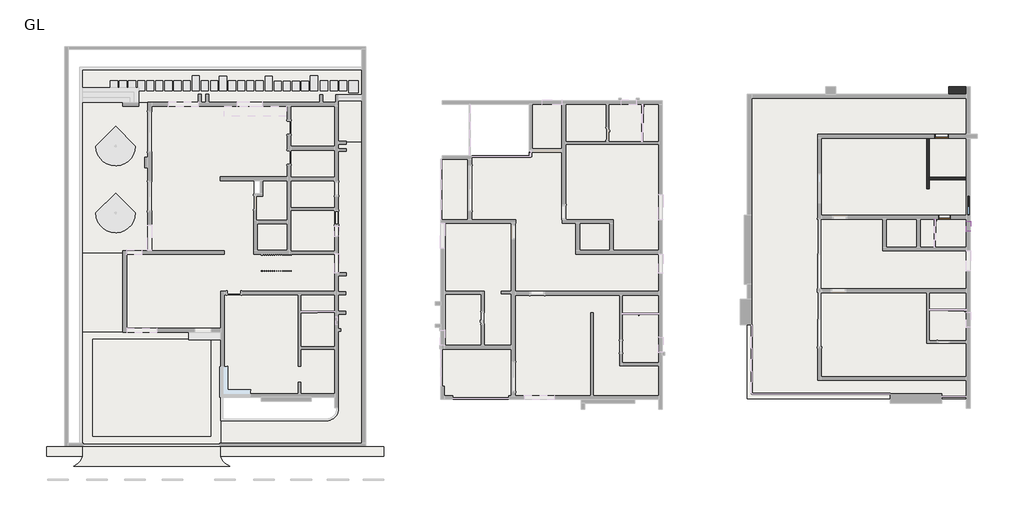
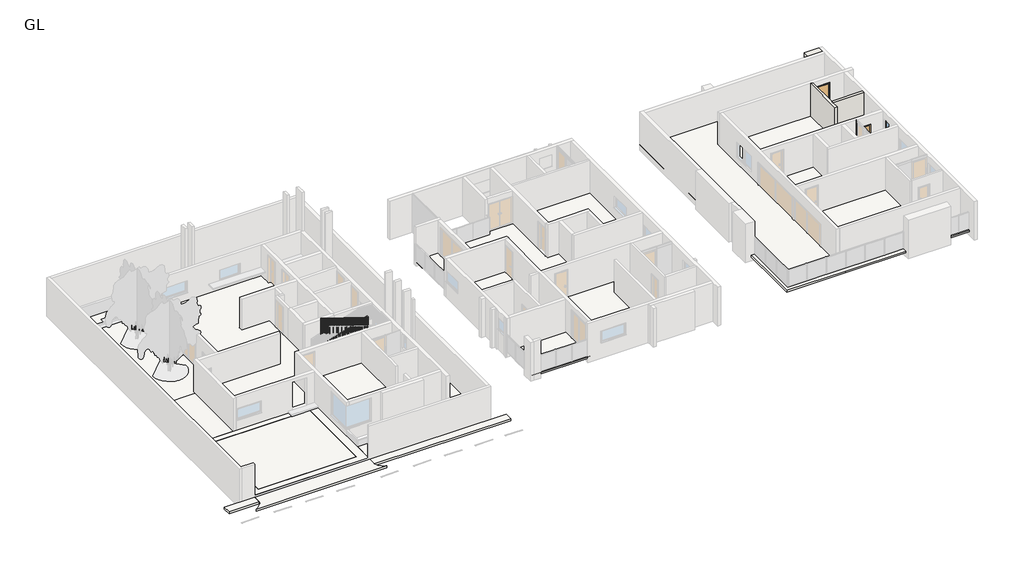
# One storey, part 5 of 6: 20 slabs, 3 walls, 2 doors, 2 members, 2 windows, 1 railing.
"""IFC4 building model written with IfcOpenShell, lengths in millimetres."""

from ifc_helpers import new_model, si_unit, point, frame, frame_2d, origin, origin_with_axes, place, context, project, spatial, polyline, circle_curve, trimmed, segment, composite_curve, outline, extrude, faceted_brep, transform, mapped, element, save
from components import door_b7cddb0a, doors_intsgl_2_5_5ac032e7, rectangular_mullion_30mm_square_28ebc8b3, rectangular_mullion_30mm_square_b4ecd99e, parametric_operable_sliding_window_6387_4_f716cbab, windows_sgl_plain_2_8d1346b0

model = new_model("IFC4")

# Units and contexts
model_context = context("Model", 3, world=origin())
ifc_project = project(units=[si_unit("LENGTHUNIT", "METRE", prefix="MILLI")], contexts=[model_context])

# Site, building, storey
site = spatial("IfcSite", under=ifc_project)
building = spatial("IfcBuilding", under=site)
storey = spatial("IfcBuildingStorey", under=building, Name="GL", Elevation=0.0)

# Doors
placement = place(None, origin())
door_shape = door_b7cddb0a(model_context)
element("IfcDoor", 1, ObjectType="Doors_IntSgl : 2'11\"", at=placement, inside=storey, context=model_context, shape_type="MappedRepresentation", body=[
    mapped(door_shape, transform((1570.3662427, 25098.2592769, 449.9570313), x_axis=(1.0, 0.0, 0.0), y_axis=(0.0, 1.0, 0.0), z_axis=(0.0, 0.0, 1.0))),
])
doors_intsgl_2_5_shape = doors_intsgl_2_5_5ac032e7(model_context)
element("IfcDoor", 2, ObjectType="Doors_IntSgl : 2.5'", at=placement, inside=storey, context=model_context, shape_type="MappedRepresentation", body=[
    mapped(doors_intsgl_2_5_shape, transform((1748.6476997, 20128.7664182, 449.9570313), x_axis=(1.0, 0.0, 0.0), y_axis=(0.0, 1.0, 0.0), z_axis=(0.0, 0.0, 1.0))),
])

# Members
rectangular_mullion_30mm_square_shape = rectangular_mullion_30mm_square_28ebc8b3(model_context)
element("IfcMember", 3, ObjectType="Rectangular Mullion : 30mm_Square", at=placement, inside=storey, context=model_context, shape_type="MappedRepresentation", body=[
    mapped(rectangular_mullion_30mm_square_shape, transform((1132.6976997, 20014.4664182, 3000.0), x_axis=(0.0, 1.0, 0.0), y_axis=(-1.0, 0.0, 0.0), z_axis=(0.0, 0.0, 1.0))),
])
rectangular_mullion_30mm_square_2_shape = rectangular_mullion_30mm_square_b4ecd99e(model_context)
element("IfcMember", 4, ObjectType="Rectangular Mullion : 30mm_Square", at=placement, inside=storey, context=model_context, shape_type="MappedRepresentation", body=[
    mapped(rectangular_mullion_30mm_square_2_shape, transform((1132.6976997, 20014.4664182, 2849.9570312), x_axis=(0.0, 1.0, 0.0), y_axis=(-1.0, 0.0, 0.0), z_axis=(0.0, 0.0, 1.0))),
])

# Railing
element("IfcRailing", 5, ObjectType="1100mm", at=placement, inside=storey, context=model_context, shape_type="SolidModel", body=[
    faceted_brep([(-40149.9681829, 16845.7531621, 1799.9767904), (-40149.9681829, 16845.7531621, 1747.4487757), (-40149.9681829, 16795.7531621, 1747.4487757), (-40149.9681829, 16795.7531621, 1799.9767904), (-36808.2681829, 16845.7531621, 2875.9675095), (-36758.2681829, 16845.7531621, 2839.538946), (-36758.2681829, 16795.7531621, 2839.538946), (-36808.2681829, 16795.7531621, 2875.9675095), (-36808.2681829, 16845.7531621, 2899.9878906), (-36758.2681829, 16845.7531621, 2849.9878906), (-36758.2681829, 16795.7531621, 2849.9878906), (-36808.2681829, 16795.7531621, 2899.9878906), (-36683.2681829, 16845.7531621, 2899.9878906), (-36683.2681829, 16845.7531621, 2849.9878906), (-36733.2681829, 16795.7531621, 2849.9878906), (-36733.2681829, 16795.7531621, 2899.9878906), (-36683.2681829, 16720.7531621, 2899.9878906), (-36683.2681829, 16720.7531621, 2849.9878906), (-36733.2681829, 16720.7531621, 2849.9878906), (-36733.2681829, 16720.7531621, 2899.9878906), (-36683.2681829, 16717.5531621, 2899.9878906), (-36683.2681829, 16667.5531621, 2849.9878906), (-36733.2681829, 16667.5531621, 2849.9878906), (-36733.2681829, 16717.5531621, 2899.9878906), (-36683.2681829, 16717.5531621, 3024.0092809), (-36683.2681829, 16667.5531621, 2974.0092809), (-36733.2681829, 16667.5531621, 2974.0092809), (-36733.2681829, 16717.5531621, 3024.0092809), (-36683.2681829, 16592.5531621, 3024.0092809), (-36683.2681829, 16592.5531621, 2974.0092809), (-36733.2681829, 16642.5531621, 2974.0092809), (-36733.2681829, 16642.5531621, 3024.0092809), (-36808.2681829, 16592.5531621, 3024.0092809), (-36816.1194278, 16592.5531621, 2974.0092809), (-36816.1194278, 16642.5531621, 2974.0092809), (-36808.2681829, 16642.5531621, 3024.0092809), (-40149.9681829, 16592.5531621, 4100.0), (-40149.9681829, 16642.5531621, 4100.0), (-40149.9681829, 16642.5531621, 4047.4719853), (-40149.9681829, 16592.5531621, 4047.4719853)], [[[0, 1, 2, 3]], [[1, 0, 4, 5]], [[2, 1, 5, 6]], [[3, 2, 6, 7]], [[0, 3, 7, 4]], [[5, 4, 8, 9]], [[6, 5, 9, 10]], [[7, 6, 10, 11]], [[4, 7, 11, 8]], [[9, 8, 12, 13]], [[10, 9, 13, 14]], [[11, 10, 14, 15]], [[8, 11, 15, 12]], [[13, 12, 16, 17]], [[14, 13, 17, 18]], [[15, 14, 18, 19]], [[12, 15, 19, 16]], [[17, 16, 20, 21]], [[18, 17, 21, 22]], [[19, 18, 22, 23]], [[16, 19, 23, 20]], [[21, 20, 24, 25]], [[22, 21, 25, 26]], [[23, 22, 26, 27]], [[20, 23, 27, 24]], [[25, 24, 28, 29]], [[26, 25, 29, 30]], [[27, 26, 30, 31]], [[24, 27, 31, 28]], [[29, 28, 32, 33]], [[30, 29, 33, 34]], [[31, 30, 34, 35]], [[28, 31, 35, 32]], [[36, 37, 38, 39]], [[33, 32, 36, 39]], [[34, 33, 39, 38]], [[35, 34, 38, 37]], [[32, 35, 37, 36]]]),
    extrude(outline(polyline([(2899.9989909, -40133.2681829), (4042.0947686, -40133.2681829), (4050.1444942, -40158.2681829), (2899.9989909, -40158.2681829), (2899.9989909, -40133.2681829)])), frame((0.0, 16605.0531621, 0.0), z_axis=(0.0, 1.0, 0.0), x_axis=(0.0, 0.0, 1.0)), (0.0, 0.0, 1.0), 25.0),
    extrude(outline(polyline([(2899.9989909, -40008.2681829), (4001.8461407, -40008.2681829), (4009.8958663, -40033.2681829), (2899.9989909, -40033.2681829), (2899.9989909, -40008.2681829)])), frame((0.0, 16605.0531621, 0.0), z_axis=(0.0, 1.0, 0.0), x_axis=(0.0, 0.0, 1.0)), (0.0, 0.0, 1.0), 25.0),
    extrude(outline(polyline([(2899.9989909, -39883.2681829), (3961.5975128, -39883.2681829), (3969.6472384, -39908.2681829), (2899.9989909, -39908.2681829), (2899.9989909, -39883.2681829)])), frame((0.0, 16605.0531621, 0.0), z_axis=(0.0, 1.0, 0.0), x_axis=(0.0, 0.0, 1.0)), (0.0, 0.0, 1.0), 25.0),
    extrude(outline(polyline([(2799.9979818, -39758.2681829), (3921.3488849, -39758.2681829), (3929.3986105, -39783.2681829), (2799.9979818, -39783.2681829), (2799.9979818, -39758.2681829)])), frame((0.0, 16605.0531621, 0.0), z_axis=(0.0, 1.0, 0.0), x_axis=(0.0, 0.0, 1.0)), (0.0, 0.0, 1.0), 25.0),
    extrude(outline(polyline([(2799.9979818, -39633.2681829), (3881.100257, -39633.2681829), (3889.1499826, -39658.2681829), (2799.9979818, -39658.2681829), (2799.9979818, -39633.2681829)])), frame((0.0, 16605.0531621, 0.0), z_axis=(0.0, 1.0, 0.0), x_axis=(0.0, 0.0, 1.0)), (0.0, 0.0, 1.0), 25.0),
    extrude(outline(polyline([(2699.9969727, -39508.2681829), (3840.8516291, -39508.2681829), (3848.9013546, -39533.2681829), (2699.9969727, -39533.2681829), (2699.9969727, -39508.2681829)])), frame((0.0, 16605.0531621, 0.0), z_axis=(0.0, 1.0, 0.0), x_axis=(0.0, 0.0, 1.0)), (0.0, 0.0, 1.0), 25.0),
    extrude(outline(polyline([(2699.9969727, -39383.2681829), (3800.6030011, -39383.2681829), (3808.6527267, -39408.2681829), (2699.9969727, -39408.2681829), (2699.9969727, -39383.2681829)])), frame((0.0, 16605.0531621, 0.0), z_axis=(0.0, 1.0, 0.0), x_axis=(0.0, 0.0, 1.0)), (0.0, 0.0, 1.0), 25.0),
    extrude(outline(polyline([(2699.9969727, -39258.2681829), (3760.3543732, -39258.2681829), (3768.4040988, -39283.2681829), (2699.9969727, -39283.2681829), (2699.9969727, -39258.2681829)])), frame((0.0, 16605.0531621, 0.0), z_axis=(0.0, 1.0, 0.0), x_axis=(0.0, 0.0, 1.0)), (0.0, 0.0, 1.0), 25.0),
    extrude(outline(polyline([(2599.9959635, -39133.2681829), (3720.1057453, -39133.2681829), (3728.1554709, -39158.2681829), (2599.9959635, -39158.2681829), (2599.9959635, -39133.2681829)])), frame((0.0, 16605.0531621, 0.0), z_axis=(0.0, 1.0, 0.0), x_axis=(0.0, 0.0, 1.0)), (0.0, 0.0, 1.0), 25.0),
    extrude(outline(polyline([(2599.9959635, -39008.2681829), (3679.8571174, -39008.2681829), (3687.906843, -39033.2681829), (2599.9959635, -39033.2681829), (2599.9959635, -39008.2681829)])), frame((0.0, 16605.0531621, 0.0), z_axis=(0.0, 1.0, 0.0), x_axis=(0.0, 0.0, 1.0)), (0.0, 0.0, 1.0), 25.0),
    extrude(outline(polyline([(2499.9949544, -38883.2681829), (3639.6084895, -38883.2681829), (3647.6582151, -38908.2681829), (2499.9949544, -38908.2681829), (2499.9949544, -38883.2681829)])), frame((0.0, 16605.0531621, 0.0), z_axis=(0.0, 1.0, 0.0), x_axis=(0.0, 0.0, 1.0)), (0.0, 0.0, 1.0), 25.0),
    extrude(outline(polyline([(2499.9949544, -38758.2681829), (3599.3598616, -38758.2681829), (3607.4095872, -38783.2681829), (2499.9949544, -38783.2681829), (2499.9949544, -38758.2681829)])), frame((0.0, 16605.0531621, 0.0), z_axis=(0.0, 1.0, 0.0), x_axis=(0.0, 0.0, 1.0)), (0.0, 0.0, 1.0), 25.0),
    extrude(outline(polyline([(2499.9949544, -38633.2681829), (3559.1112337, -38633.2681829), (3567.1609593, -38658.2681829), (2499.9949544, -38658.2681829), (2499.9949544, -38633.2681829)])), frame((0.0, 16605.0531621, 0.0), z_axis=(0.0, 1.0, 0.0), x_axis=(0.0, 0.0, 1.0)), (0.0, 0.0, 1.0), 25.0),
    extrude(outline(polyline([(2399.9939453, -38508.2681829), (3518.8626058, -38508.2681829), (3526.9123314, -38533.2681829), (2399.9939453, -38533.2681829), (2399.9939453, -38508.2681829)])), frame((0.0, 16605.0531621, 0.0), z_axis=(0.0, 1.0, 0.0), x_axis=(0.0, 0.0, 1.0)), (0.0, 0.0, 1.0), 25.0),
    extrude(outline(polyline([(2399.9939453, -38383.2681829), (3478.6139779, -38383.2681829), (3486.6637034, -38408.2681829), (2399.9939453, -38408.2681829), (2399.9939453, -38383.2681829)])), frame((0.0, 16605.0531621, 0.0), z_axis=(0.0, 1.0, 0.0), x_axis=(0.0, 0.0, 1.0)), (0.0, 0.0, 1.0), 25.0),
    extrude(outline(polyline([(2299.9929362, -38258.2681829), (3438.36535, -38258.2681829), (3446.4150755, -38283.2681829), (2299.9929362, -38283.2681829), (2299.9929362, -38258.2681829)])), frame((0.0, 16605.0531621, 0.0), z_axis=(0.0, 1.0, 0.0), x_axis=(0.0, 0.0, 1.0)), (0.0, 0.0, 1.0), 25.0),
    extrude(outline(polyline([(2299.9929362, -38133.2681829), (3398.116722, -38133.2681829), (3406.1664476, -38158.2681829), (2299.9929362, -38158.2681829), (2299.9929362, -38133.2681829)])), frame((0.0, 16605.0531621, 0.0), z_axis=(0.0, 1.0, 0.0), x_axis=(0.0, 0.0, 1.0)), (0.0, 0.0, 1.0), 25.0),
    extrude(outline(polyline([(2299.9929362, -38008.2681829), (3357.8680941, -38008.2681829), (3365.9178197, -38033.2681829), (2299.9929362, -38033.2681829), (2299.9929362, -38008.2681829)])), frame((0.0, 16605.0531621, 0.0), z_axis=(0.0, 1.0, 0.0), x_axis=(0.0, 0.0, 1.0)), (0.0, 0.0, 1.0), 25.0),
    extrude(outline(polyline([(2199.9919271, -37883.2681829), (3317.6194662, -37883.2681829), (3325.6691918, -37908.2681829), (2199.9919271, -37908.2681829), (2199.9919271, -37883.2681829)])), frame((0.0, 16605.0531621, 0.0), z_axis=(0.0, 1.0, 0.0), x_axis=(0.0, 0.0, 1.0)), (0.0, 0.0, 1.0), 25.0),
    extrude(outline(polyline([(2199.9919271, -37758.2681829), (3277.3708383, -37758.2681829), (3285.4205639, -37783.2681829), (2199.9919271, -37783.2681829), (2199.9919271, -37758.2681829)])), frame((0.0, 16605.0531621, 0.0), z_axis=(0.0, 1.0, 0.0), x_axis=(0.0, 0.0, 1.0)), (0.0, 0.0, 1.0), 25.0),
    extrude(outline(polyline([(2099.990918, -37633.2681829), (3237.1222104, -37633.2681829), (3245.171936, -37658.2681829), (2099.990918, -37658.2681829), (2099.990918, -37633.2681829)])), frame((0.0, 16605.0531621, 0.0), z_axis=(0.0, 1.0, 0.0), x_axis=(0.0, 0.0, 1.0)), (0.0, 0.0, 1.0), 25.0),
    extrude(outline(polyline([(2099.990918, -37508.2681829), (3196.8735825, -37508.2681829), (3204.9233081, -37533.2681829), (2099.990918, -37533.2681829), (2099.990918, -37508.2681829)])), frame((0.0, 16605.0531621, 0.0), z_axis=(0.0, 1.0, 0.0), x_axis=(0.0, 0.0, 1.0)), (0.0, 0.0, 1.0), 25.0),
    extrude(outline(polyline([(2099.990918, -37383.2681829), (3156.6249546, -37383.2681829), (3164.6746802, -37408.2681829), (2099.990918, -37408.2681829), (2099.990918, -37383.2681829)])), frame((0.0, 16605.0531621, 0.0), z_axis=(0.0, 1.0, 0.0), x_axis=(0.0, 0.0, 1.0)), (0.0, 0.0, 1.0), 25.0),
    extrude(outline(polyline([(1999.9899089, -37258.2681829), (3116.3763267, -37258.2681829), (3124.4260522, -37283.2681829), (1999.9899089, -37283.2681829), (1999.9899089, -37258.2681829)])), frame((0.0, 16605.0531621, 0.0), z_axis=(0.0, 1.0, 0.0), x_axis=(0.0, 0.0, 1.0)), (0.0, 0.0, 1.0), 25.0),
    extrude(outline(polyline([(1999.9899089, -37133.2681829), (3076.1276988, -37133.2681829), (3084.1774243, -37158.2681829), (1999.9899089, -37158.2681829), (1999.9899089, -37133.2681829)])), frame((0.0, 16605.0531621, 0.0), z_axis=(0.0, 1.0, 0.0), x_axis=(0.0, 0.0, 1.0)), (0.0, 0.0, 1.0), 25.0),
    extrude(outline(polyline([(1899.9888997, -37008.2681829), (3035.8790708, -37008.2681829), (3043.9287964, -37033.2681829), (1899.9888997, -37033.2681829), (1899.9888997, -37008.2681829)])), frame((0.0, 16605.0531621, 0.0), z_axis=(0.0, 1.0, 0.0), x_axis=(0.0, 0.0, 1.0)), (0.0, 0.0, 1.0), 25.0),
    extrude(outline(polyline([(1899.9888997, -36883.2681829), (2995.6304429, -36883.2681829), (3003.6801685, -36908.2681829), (1899.9888997, -36908.2681829), (1899.9888997, -36883.2681829)])), frame((0.0, 16605.0531621, 0.0), z_axis=(0.0, 1.0, 0.0), x_axis=(0.0, 0.0, 1.0)), (0.0, 0.0, 1.0), 25.0),
    extrude(outline(polyline([(-36758.2681829, 16630.0531621), (-36758.2681829, 16605.0531621), (-36783.2681829, 16605.0531621), (-36783.2681829, 16630.0531621), (-36758.2681829, 16630.0531621)])), frame((0.0, 0.0, 1899.9888997), z_axis=(0.0, 0.0, 1.0), x_axis=(1.0, 0.0, 0.0)), (0.0, 0.0, 1.0), 1074.0203811),
    extrude(outline(polyline([(-36720.7681829, 16645.7531621), (-36695.7681829, 16645.7531621), (-36695.7681829, 16620.7531621), (-36720.7681829, 16620.7531621), (-36720.7681829, 16645.7531621)])), frame((0.0, 0.0, 1799.9878906), z_axis=(0.0, 0.0, 1.0), x_axis=(1.0, 0.0, 0.0)), (0.0, 0.0, 1.0), 1174.0213903),
    extrude(outline(polyline([(-36720.7681829, 16770.7531621), (-36695.7681829, 16770.7531621), (-36695.7681829, 16745.7531621), (-36720.7681829, 16745.7531621), (-36720.7681829, 16770.7531621)])), frame((0.0, 0.0, 1799.9878906), z_axis=(0.0, 0.0, 1.0), x_axis=(1.0, 0.0, 0.0)), (0.0, 0.0, 1.0), 1050.0),
    extrude(outline(polyline([(-36724.9681829, 16808.2531621), (-36724.9681829, 16833.2531621), (-36699.9681829, 16833.2531621), (-36699.9681829, 16808.2531621), (-36724.9681829, 16808.2531621)])), frame((0.0, 0.0, 1799.9878906), z_axis=(0.0, 0.0, 1.0), x_axis=(1.0, 0.0, 0.0)), (0.0, 0.0, 1.0), 1050.0),
    extrude(outline(polyline([(2810.0125525, -36849.9681829), (1699.9868815, -36849.9681829), (1699.9868815, -36824.9681829), (2818.0622781, -36824.9681829), (2810.0125525, -36849.9681829)])), frame((0.0, 16808.2531621, 0.0), z_axis=(0.0, 1.0, 0.0), x_axis=(0.0, 0.0, 1.0)), (0.0, 0.0, 1.0), 25.0),
    extrude(outline(polyline([(2769.7639246, -36974.9681829), (1699.9868815, -36974.9681829), (1699.9868815, -36949.9681829), (2777.8136502, -36949.9681829), (2769.7639246, -36974.9681829)])), frame((0.0, 16808.2531621, 0.0), z_axis=(0.0, 1.0, 0.0), x_axis=(0.0, 0.0, 1.0)), (0.0, 0.0, 1.0), 25.0),
    extrude(outline(polyline([(2729.5152967, -37099.9681829), (1599.9858724, -37099.9681829), (1599.9858724, -37074.9681829), (2737.5650223, -37074.9681829), (2729.5152967, -37099.9681829)])), frame((0.0, 16808.2531621, 0.0), z_axis=(0.0, 1.0, 0.0), x_axis=(0.0, 0.0, 1.0)), (0.0, 0.0, 1.0), 25.0),
    extrude(outline(polyline([(2689.2666688, -37224.9681829), (1599.9858724, -37224.9681829), (1599.9858724, -37199.9681829), (2697.3163944, -37199.9681829), (2689.2666688, -37224.9681829)])), frame((0.0, 16808.2531621, 0.0), z_axis=(0.0, 1.0, 0.0), x_axis=(0.0, 0.0, 1.0)), (0.0, 0.0, 1.0), 25.0),
    extrude(outline(polyline([(2649.0180409, -37349.9681829), (1599.9858724, -37349.9681829), (1599.9858724, -37324.9681829), (2657.0677665, -37324.9681829), (2649.0180409, -37349.9681829)])), frame((0.0, 16808.2531621, 0.0), z_axis=(0.0, 1.0, 0.0), x_axis=(0.0, 0.0, 1.0)), (0.0, 0.0, 1.0), 25.0),
    extrude(outline(polyline([(2608.769413, -37474.9681829), (1499.9848633, -37474.9681829), (1499.9848633, -37449.9681829), (2616.8191385, -37449.9681829), (2608.769413, -37474.9681829)])), frame((0.0, 16808.2531621, 0.0), z_axis=(0.0, 1.0, 0.0), x_axis=(0.0, 0.0, 1.0)), (0.0, 0.0, 1.0), 25.0),
    extrude(outline(polyline([(2568.5207851, -37599.9681829), (1499.9848633, -37599.9681829), (1499.9848633, -37574.9681829), (2576.5705106, -37574.9681829), (2568.5207851, -37599.9681829)])), frame((0.0, 16808.2531621, 0.0), z_axis=(0.0, 1.0, 0.0), x_axis=(0.0, 0.0, 1.0)), (0.0, 0.0, 1.0), 25.0),
    extrude(outline(polyline([(2528.2721571, -37724.9681829), (1399.9838542, -37724.9681829), (1399.9838542, -37699.9681829), (2536.3218827, -37699.9681829), (2528.2721571, -37724.9681829)])), frame((0.0, 16808.2531621, 0.0), z_axis=(0.0, 1.0, 0.0), x_axis=(0.0, 0.0, 1.0)), (0.0, 0.0, 1.0), 25.0),
    extrude(outline(polyline([(2488.0235292, -37849.9681829), (1399.9838542, -37849.9681829), (1399.9838542, -37824.9681829), (2496.0732548, -37824.9681829), (2488.0235292, -37849.9681829)])), frame((0.0, 16808.2531621, 0.0), z_axis=(0.0, 1.0, 0.0), x_axis=(0.0, 0.0, 1.0)), (0.0, 0.0, 1.0), 25.0),
    extrude(outline(polyline([(2447.7749013, -37974.9681829), (1399.9838542, -37974.9681829), (1399.9838542, -37949.9681829), (2455.8246269, -37949.9681829), (2447.7749013, -37974.9681829)])), frame((0.0, 16808.2531621, 0.0), z_axis=(0.0, 1.0, 0.0), x_axis=(0.0, 0.0, 1.0)), (0.0, 0.0, 1.0), 25.0),
    extrude(outline(polyline([(2407.5262734, -38099.9681829), (1299.9828451, -38099.9681829), (1299.9828451, -38074.9681829), (2415.575999, -38074.9681829), (2407.5262734, -38099.9681829)])), frame((0.0, 16808.2531621, 0.0), z_axis=(0.0, 1.0, 0.0), x_axis=(0.0, 0.0, 1.0)), (0.0, 0.0, 1.0), 25.0),
    extrude(outline(polyline([(2367.2776455, -38224.9681829), (1299.9828451, -38224.9681829), (1299.9828451, -38199.9681829), (2375.3273711, -38199.9681829), (2367.2776455, -38224.9681829)])), frame((0.0, 16808.2531621, 0.0), z_axis=(0.0, 1.0, 0.0), x_axis=(0.0, 0.0, 1.0)), (0.0, 0.0, 1.0), 25.0),
    extrude(outline(polyline([(2327.0290176, -38349.9681829), (1199.9818359, -38349.9681829), (1199.9818359, -38324.9681829), (2335.0787432, -38324.9681829), (2327.0290176, -38349.9681829)])), frame((0.0, 16808.2531621, 0.0), z_axis=(0.0, 1.0, 0.0), x_axis=(0.0, 0.0, 1.0)), (0.0, 0.0, 1.0), 25.0),
    extrude(outline(polyline([(2286.7803897, -38474.9681829), (1199.9818359, -38474.9681829), (1199.9818359, -38449.9681829), (2294.8301153, -38449.9681829), (2286.7803897, -38474.9681829)])), frame((0.0, 16808.2531621, 0.0), z_axis=(0.0, 1.0, 0.0), x_axis=(0.0, 0.0, 1.0)), (0.0, 0.0, 1.0), 25.0),
    extrude(outline(polyline([(2246.5317618, -38599.9681829), (1199.9818359, -38599.9681829), (1199.9818359, -38574.9681829), (2254.5814873, -38574.9681829), (2246.5317618, -38599.9681829)])), frame((0.0, 16808.2531621, 0.0), z_axis=(0.0, 1.0, 0.0), x_axis=(0.0, 0.0, 1.0)), (0.0, 0.0, 1.0), 25.0),
    extrude(outline(polyline([(2206.2831339, -38724.9681829), (1099.9808268, -38724.9681829), (1099.9808268, -38699.9681829), (2214.3328594, -38699.9681829), (2206.2831339, -38724.9681829)])), frame((0.0, 16808.2531621, 0.0), z_axis=(0.0, 1.0, 0.0), x_axis=(0.0, 0.0, 1.0)), (0.0, 0.0, 1.0), 25.0),
    extrude(outline(polyline([(2166.0345059, -38849.9681829), (1099.9808268, -38849.9681829), (1099.9808268, -38824.9681829), (2174.0842315, -38824.9681829), (2166.0345059, -38849.9681829)])), frame((0.0, 16808.2531621, 0.0), z_axis=(0.0, 1.0, 0.0), x_axis=(0.0, 0.0, 1.0)), (0.0, 0.0, 1.0), 25.0),
    extrude(outline(polyline([(2125.785878, -38974.9681829), (999.9798177, -38974.9681829), (999.9798177, -38949.9681829), (2133.8356036, -38949.9681829), (2125.785878, -38974.9681829)])), frame((0.0, 16808.2531621, 0.0), z_axis=(0.0, 1.0, 0.0), x_axis=(0.0, 0.0, 1.0)), (0.0, 0.0, 1.0), 25.0),
    extrude(outline(polyline([(2085.5372501, -39099.9681829), (999.9798177, -39099.9681829), (999.9798177, -39074.9681829), (2093.5869757, -39074.9681829), (2085.5372501, -39099.9681829)])), frame((0.0, 16808.2531621, 0.0), z_axis=(0.0, 1.0, 0.0), x_axis=(0.0, 0.0, 1.0)), (0.0, 0.0, 1.0), 25.0),
    extrude(outline(polyline([(2045.2886222, -39224.9681829), (999.9798177, -39224.9681829), (999.9798177, -39199.9681829), (2053.3383478, -39199.9681829), (2045.2886222, -39224.9681829)])), frame((0.0, 16808.2531621, 0.0), z_axis=(0.0, 1.0, 0.0), x_axis=(0.0, 0.0, 1.0)), (0.0, 0.0, 1.0), 25.0),
    extrude(outline(polyline([(2005.0399943, -39349.9681829), (899.9788086, -39349.9681829), (899.9788086, -39324.9681829), (2013.0897199, -39324.9681829), (2005.0399943, -39349.9681829)])), frame((0.0, 16808.2531621, 0.0), z_axis=(0.0, 1.0, 0.0), x_axis=(0.0, 0.0, 1.0)), (0.0, 0.0, 1.0), 25.0),
    extrude(outline(polyline([(1964.7913664, -39474.9681829), (899.9788086, -39474.9681829), (899.9788086, -39449.9681829), (1972.841092, -39449.9681829), (1964.7913664, -39474.9681829)])), frame((0.0, 16808.2531621, 0.0), z_axis=(0.0, 1.0, 0.0), x_axis=(0.0, 0.0, 1.0)), (0.0, 0.0, 1.0), 25.0),
    extrude(outline(polyline([(1924.5427385, -39599.9681829), (799.9777995, -39599.9681829), (799.9777995, -39574.9681829), (1932.5924641, -39574.9681829), (1924.5427385, -39599.9681829)])), frame((0.0, 16808.2531621, 0.0), z_axis=(0.0, 1.0, 0.0), x_axis=(0.0, 0.0, 1.0)), (0.0, 0.0, 1.0), 25.0),
    extrude(outline(polyline([(1884.2941106, -39724.9681829), (799.9777995, -39724.9681829), (799.9777995, -39699.9681829), (1892.3438361, -39699.9681829), (1884.2941106, -39724.9681829)])), frame((0.0, 16808.2531621, 0.0), z_axis=(0.0, 1.0, 0.0), x_axis=(0.0, 0.0, 1.0)), (0.0, 0.0, 1.0), 25.0),
    extrude(outline(polyline([(1844.0454827, -39849.9681829), (799.9777995, -39849.9681829), (799.9777995, -39824.9681829), (1852.0952082, -39824.9681829), (1844.0454827, -39849.9681829)])), frame((0.0, 16808.2531621, 0.0), z_axis=(0.0, 1.0, 0.0), x_axis=(0.0, 0.0, 1.0)), (0.0, 0.0, 1.0), 25.0),
    extrude(outline(polyline([(1803.7968547, -39974.9681829), (699.9767904, -39974.9681829), (699.9767904, -39949.9681829), (1811.8465803, -39949.9681829), (1803.7968547, -39974.9681829)])), frame((0.0, 16808.2531621, 0.0), z_axis=(0.0, 1.0, 0.0), x_axis=(0.0, 0.0, 1.0)), (0.0, 0.0, 1.0), 25.0),
    extrude(outline(polyline([(1763.5482268, -40099.9681829), (699.9767904, -40099.9681829), (699.9767904, -40074.9681829), (1771.5979524, -40074.9681829), (1763.5482268, -40099.9681829)])), frame((0.0, 16808.2531621, 0.0), z_axis=(0.0, 1.0, 0.0), x_axis=(0.0, 0.0, 1.0)), (0.0, 0.0, 1.0), 25.0),
    extrude(outline(polyline([(-36720.7681829, 16630.0531621), (-36695.7681829, 16630.0531621), (-36695.7681829, 16605.0531621), (-36720.7681829, 16605.0531621), (-36720.7681829, 16630.0531621)])), frame((0.0, 0.0, 1799.9878906), z_axis=(0.0, 0.0, 1.0), x_axis=(1.0, 0.0, 0.0)), (0.0, 0.0, 1.0), 1174.0213903),
    extrude(outline(polyline([(-36720.7681829, 16808.2531621), (-36720.7681829, 16833.2531621), (-36695.7681829, 16833.2531621), (-36695.7681829, 16808.2531621), (-36720.7681829, 16808.2531621)])), frame((0.0, 0.0, 1799.9878906), z_axis=(0.0, 0.0, 1.0), x_axis=(1.0, 0.0, 0.0)), (0.0, 0.0, 1.0), 1050.0),
    extrude(outline(polyline([(2899.9989909, -40124.9681829), (4039.4222597, -40124.9681829), (4047.4719853, -40149.9681829), (2899.9989909, -40149.9681829), (2899.9989909, -40124.9681829)])), frame((0.0, 16605.0531621, 0.0), z_axis=(0.0, 1.0, 0.0), x_axis=(0.0, 0.0, 1.0)), (0.0, 0.0, 1.0), 25.0),
    extrude(outline(polyline([(1747.4487757, -40149.9681829), (699.9767904, -40149.9681829), (699.9767904, -40124.9681829), (1755.4985013, -40124.9681829), (1747.4487757, -40149.9681829)])), frame((0.0, 16808.2531621, 0.0), z_axis=(0.0, 1.0, 0.0), x_axis=(0.0, 0.0, 1.0)), (0.0, 0.0, 1.0), 25.0),
])

# Slabs
element("IfcSlab", 6, at=placement, inside=storey, context=model_context, shape_type="SweptSolid", body=[
    extrude(outline(polyline([(-35460.84796, 20543.2041063), (-35460.84796, 18041.3041063), (-38343.74796, 18041.3041063), (-38343.74796, 20543.2041063), (-35460.84796, 20543.2041063)])), frame((0.0, 0.0, 449.9570312), z_axis=(0.0, 0.0, 1.0), x_axis=(1.0, 0.0, 0.0)), (0.0, 0.0, 1.0), 150.01875),
])
element("IfcSlab", 7, at=placement, inside=storey, context=model_context, shape_type="SweptSolid", body=[
    extrude(outline(polyline([(-43267.3417659, 12654.8361345), (-43267.3417659, 6711.2361345), (-50480.9417659, 6711.2361345), (-50480.9417659, 12654.8361345), (-43267.3417659, 12654.8361345)])), frame((0.0, 0.0, 299.9382813), z_axis=(0.0, 0.0, 1.0), x_axis=(1.0, 0.0, 0.0)), (0.0, 0.0, 1.0), 150.01875),
])
element("IfcSlab", 8, at=placement, inside=storey, context=model_context, shape_type="SweptSolid", body=[
    extrude(outline(polyline([(-42650.6472522, 13078.7799463), (-42650.6472522, 6250.4436329), (-51132.7755215, 6250.4436329), (-51132.7755215, 13078.7799463), (-42650.6472522, 13078.7799463)]), holes=[polyline([(-50480.9417659, 6711.2361345), (-43267.3417659, 6711.2361345), (-43267.3417659, 12654.8361345), (-50480.9417659, 12654.8361345), (-50480.9417659, 6711.2361345)])]), frame((0.0, 0.0, 299.9382813), z_axis=(0.0, 0.0, 1.0), x_axis=(1.0, 0.0, 0.0)), (0.0, 0.0, 1.0), 150.01875),
])
element("IfcSlab", 9, at=placement, inside=storey, context=model_context, shape_type="SweptSolid", body=[
    extrude(outline(polyline([(-32643.0472522, 6059.9436329), (-32643.0472522, 5475.7436329), (-42650.6472522, 5475.7436329), (-42650.6472522, 6059.9436329), (-32643.0472522, 6059.9436329)])), frame((0.0, 0.0, 299.9382813), z_axis=(0.0, 0.0, 1.0), x_axis=(1.0, 0.0, 0.0)), (0.0, 0.0, 1.0), 150.01875),
    extrude(outline(polyline([(-51119.9445457, 6056.3234693), (-51119.9445457, 5472.1234693), (-53329.7445457, 5472.1234693), (-53329.7445457, 6056.3234693), (-51119.9445457, 6056.3234693)])), frame((0.0, 0.0, 299.9382813), z_axis=(0.0, 0.0, 1.0), x_axis=(1.0, 0.0, 0.0)), (0.0, 0.0, 1.0), 150.01875),
])
element("IfcSlab", 10, at=placement, inside=storey, context=model_context, shape_type="SweptSolid", body=[
    extrude(outline(composite_curve([segment(polyline([(-42661.7445457, 6056.3234693), (-42661.7445457, 5475.7436329)]), True, "CONTINUOUS"), segment(trimmed(circle_curve(frame_2d((-41816.6571051, 5698.3835361)), 873.9229421), [point((-42661.7445457, 5475.7436329))], [point((-42093.5791975, 4869.4954474))], True, "CARTESIAN"), True, "CONTINUOUS"), segment(polyline([(-42093.5791975, 4869.4954474), (-51669.3791975, 4869.4954474)]), True, "CONTINUOUS"), segment(trimmed(circle_curve(frame_2d((-52005.8369926, 5728.0367654)), 922.1155257), [point((-51669.3791975, 4869.4954474))], [point((-51119.9445457, 5472.1234693))], True, "CARTESIAN"), True, "CONTINUOUS"), segment(polyline([(-51119.9445457, 5472.1234693), (-51119.9445457, 6056.3234693), (-42661.7445457, 6056.3234693)]), True, "CONTINUOUS")], self_intersect=False)), frame((0.0, 0.0, 299.9382813), z_axis=(0.0, 0.0, 1.0), x_axis=(1.0, 0.0, 0.0)), (0.0, 0.0, 1.0), 150.01875),
])
element("IfcSlab", 11, at=placement, inside=storey, context=model_context, shape_type="SweptSolid", body=[
    extrude(outline(polyline([(-33990.9791975, 29177.2755965), (-33990.9791975, 27628.0855094), (-35422.74796, 27628.0855094), (-35422.74796, 27163.0621553), (-51132.7755215, 27163.0621553), (-51132.7755215, 29177.2755965), (-33990.9791975, 29177.2755965)])), frame((0.0, 0.0, -145.0578125), z_axis=(0.0, 0.0, 1.0), x_axis=(1.0, 0.0, 0.0)), (0.0, 0.0, 1.0), 150.01875),
])
element("IfcSlab", 12, ObjectType="DECK", at=placement, inside=storey, context=model_context, shape_type="SweptSolid", body=[
    extrude(outline(polyline([(-47116.4786333, 27163.7616741), (-47116.4786333, 17927.077827), (-51132.7755215, 17927.077827), (-51132.7755215, 27163.7616741), (-47116.4786333, 27163.7616741)])), frame((0.0, 0.0, 299.9382813), z_axis=(0.0, 0.0, 1.0), x_axis=(1.0, 0.0, 0.0)), (0.0, 0.0, 1.0), 150.01875),
])
element("IfcSlab", 13, ObjectType="LIFT FLOOR", at=placement, inside=storey, context=model_context, shape_type="SweptSolid", body=[
    extrude(outline(polyline([(-38572.34796, 19730.4041063), (-38572.34796, 18092.1041063), (-40401.14796, 18092.1041063), (-40401.14796, 19730.4041063), (-38572.34796, 19730.4041063)])), frame((0.0, 0.0, 449.9570312), z_axis=(0.0, 0.0, 1.0), x_axis=(1.0, 0.0, 0.0)), (0.0, 0.0, 1.0), 150.01875),
    extrude(outline(polyline([(-33990.9791975, 27239.2621553), (-33990.9791975, 24746.9041063), (-35422.74796, 24746.9041063), (-35422.74796, 27239.2621553), (-33990.9791975, 27239.2621553)])), frame((0.0, 0.0, 449.9570312), z_axis=(0.0, 0.0, 1.0), x_axis=(1.0, 0.0, 0.0)), (0.0, 0.0, 1.0), 150.01875),
])
element("IfcSlab", 14, ObjectType="LIFT FLOOR", at=placement, inside=storey, context=model_context, shape_type="SweptSolid", body=[
    extrude(outline(polyline([(-18782.3556238, 19772.273283), (-18782.3556238, 18095.873283), (-20636.5556238, 18095.873283), (-20636.5556238, 19772.273283), (-18782.3556238, 19772.273283)])), frame((0.0, 0.0, 299.9382813), z_axis=(0.0, 0.0, 1.0), x_axis=(1.0, 0.0, 0.0)), (0.0, 0.0, 1.0), 150.01875),
])
element("IfcSlab", 15, ObjectType="LIFT FLOOR", at=placement, inside=storey, context=model_context, shape_type="SweptSolid", body=[
    extrude(outline(polyline([(40.4976997, 20014.4664182), (40.4976997, 18298.634827), (-1813.7023003, 18298.634827), (-1813.7023003, 20014.4664182), (40.4976997, 20014.4664182)])), frame((0.0, 0.0, 299.9382813), z_axis=(0.0, 0.0, 1.0), x_axis=(1.0, 0.0, 0.0)), (0.0, 0.0, 1.0), 150.01875),
])
element("IfcSlab", 16, ObjectType="OPEN TERRACE", at=placement, inside=storey, context=model_context, shape_type="SweptSolid", body=[
    extrude(outline(polyline([(-6036.9337573, 9008.1341759), (-10342.6061453, 9008.1341759), (-10342.6061453, 27687.1795779), (-6036.9337573, 27687.1795779), (3323.4476997, 27687.1795779), (3323.4476997, 25212.5592769), (-6036.9337573, 25212.5592769), (-6036.9337573, 10124.9592769), (3056.2662427, 10124.9592769), (3056.2662427, 9008.1341759), (-6036.9337573, 9008.1341759)])), frame((0.0, 0.0, 299.9382813), z_axis=(0.0, 0.0, 1.0), x_axis=(1.0, 0.0, 0.0)), (0.0, 0.0, 1.0), 150.01875),
])
element("IfcSlab", 17, ObjectType="OUTDOOR", at=placement, inside=storey, context=model_context, shape_type="SweptSolid", body=[
    extrude(outline(polyline([(-48640.4786333, 17927.077827), (-48640.4786333, 13078.7799463), (-51132.7755215, 13078.7799463), (-51132.7755215, 17927.077827), (-48640.4786333, 17927.077827)])), frame((0.0, 0.0, 299.9382813), z_axis=(0.0, 0.0, 1.0), x_axis=(1.0, 0.0, 0.0)), (0.0, 0.0, 1.0), 150.01875),
    extrude(outline(composite_curve([segment(polyline([(-33990.9791975, 24746.9041063), (-33990.9791975, 6266.0065956), (-34996.6580817, 6266.0065956), (-42641.0383946, 6266.0065956), (-42641.0383946, 7643.9408146), (-36062.4383946, 7643.9408146)]), True, "CONTINUOUS"), segment(trimmed(circle_curve(frame_2d((-36238.0484419, 8440.1041063)), 815.3004819), [point((-36062.4383946, 7643.9408146))], [point((-35422.74796, 8440.1041063))], True, "CARTESIAN"), True, "CONTINUOUS"), segment(polyline([(-35422.74796, 8440.1041063), (-35422.74796, 24746.9041063), (-33990.9791975, 24746.9041063)]), True, "CONTINUOUS")], self_intersect=False)), frame((0.0, 0.0, 299.9382813), z_axis=(0.0, 0.0, 1.0), x_axis=(1.0, 0.0, 0.0)), (0.0, 0.0, 1.0), 150.01875),
])
element("IfcSlab", 18, ObjectType="TOILET", at=placement, inside=storey, context=model_context, shape_type="SweptSolid", body=[
    extrude(outline(polyline([(-35651.34796, 22372.0041063), (-35651.34796, 20721.0041063), (-38343.74796, 20721.0041063), (-38343.74796, 22372.0041063), (-35651.34796, 22372.0041063)])), frame((0.0, 0.0, 449.9570312), z_axis=(0.0, 0.0, 1.0), x_axis=(1.0, 0.0, 0.0)), (0.0, 0.0, 1.0), 150.01875),
    extrude(outline(polyline([(-38572.34796, 19959.0041063), (-40477.34796, 19959.0041063), (-40477.34796, 21432.2041063), (-40070.94796, 21432.2041063), (-40070.94796, 22359.3041063), (-38572.34796, 22359.3041063), (-38572.34796, 19959.0041063)])), frame((0.0, 0.0, 449.9570312), z_axis=(0.0, 0.0, 1.0), x_axis=(1.0, 0.0, 0.0)), (0.0, 0.0, 1.0), 150.01875),
    extrude(outline(polyline([(-35651.34796, 15374.3041063), (-35651.34796, 12199.3041063), (-37740.3080191, 12199.3041063), (-37740.3080191, 15374.3041063), (-35651.34796, 15374.3041063)])), frame((0.0, 0.0, 449.9570312), z_axis=(0.0, 0.0, 1.0), x_axis=(1.0, 0.0, 0.0)), (0.0, 0.0, 1.0), 150.01875),
])
element("IfcSlab", 19, ObjectType="TOILET", at=placement, inside=storey, context=model_context, shape_type="SweptSolid", body=[
    extrude(outline(polyline([(-15785.8464553, 27046.1107151), (-15785.8464553, 24760.1107151), (-18859.2464553, 24760.1107151), (-18859.2464553, 27046.1107151), (-15785.8464553, 27046.1107151)])), frame((0.0, 0.0, 299.9382813), z_axis=(0.0, 0.0, 1.0), x_axis=(1.0, 0.0, 0.0)), (0.0, 0.0, 1.0), 150.01875),
    extrude(outline(polyline([(-15791.6562878, 15334.8726609), (-15791.6562878, 11194.6726609), (-18026.8562878, 11194.6726609), (-18026.8562878, 15334.8726609), (-15791.6562878, 15334.8726609)])), frame((0.0, 0.0, 299.9382813), z_axis=(0.0, 0.0, 1.0), x_axis=(1.0, 0.0, 0.0)), (0.0, 0.0, 1.0), 150.01875),
    extrude(outline(polyline([(-26687.7458397, 15445.3525128), (-26687.7458397, 12270.3525128), (-28846.7458397, 12270.3525128), (-28846.7458397, 15445.3525128), (-26687.7458397, 15445.3525128)])), frame((0.0, 0.0, 299.9382813), z_axis=(0.0, 0.0, 1.0), x_axis=(1.0, 0.0, 0.0)), (0.0, 0.0, 1.0), 150.01875),
])
element("IfcSlab", 20, ObjectType="TOILET", at=placement, inside=storey, context=model_context, shape_type="SweptSolid", body=[
    extrude(outline(polyline([(3094.8476997, 15506.9220058), (3094.8476997, 12560.5220058), (807.7626485, 12560.5220058), (807.7626485, 15506.9220058), (3094.8476997, 15506.9220058)])), frame((0.0, 0.0, 299.9382813), z_axis=(0.0, 0.0, 1.0), x_axis=(1.0, 0.0, 0.0)), (0.0, 0.0, 1.0), 150.01875),
    extrude(outline(polyline([(3094.8476997, 20014.4664182), (3094.8476997, 18298.634827), (269.0976997, 18298.634827), (269.0976997, 20014.4664182), (3094.8476997, 20014.4664182)])), frame((0.0, 0.0, 299.9382813), z_axis=(0.0, 0.0, 1.0), x_axis=(1.0, 0.0, 0.0)), (0.0, 0.0, 1.0), 150.01875),
])
element("IfcSlab", 21, ObjectType="WIDE BALCONY FLOOR", at=placement, inside=storey, context=model_context, shape_type="SweptSolid", body=[
    extrude(outline(polyline([(-29043.9556238, 19746.873283), (-29043.9556238, 23887.073283), (-27265.9556238, 23887.073283), (-27265.9556238, 19746.873283), (-29043.9556238, 19746.873283)])), frame((0.0, 0.0, 299.9382813), z_axis=(0.0, 0.0, 1.0), x_axis=(1.0, 0.0, 0.0)), (0.0, 0.0, 1.0), 150.01875),
    extrude(outline(polyline([(-29035.2875606, 12018.7346755), (-24818.8875606, 12018.7346755), (-24818.8875606, 8970.7346755), (-29035.2875606, 8970.7346755), (-29035.2875606, 12018.7346755)])), frame((0.0, 0.0, 299.9382813), z_axis=(0.0, 0.0, 1.0), x_axis=(1.0, 0.0, 0.0)), (0.0, 0.0, 1.0), 150.01875),
])
element("IfcSlab", 22, ObjectType="inner main", at=placement, inside=storey, context=model_context, shape_type="SweptSolid", body=[
    extrude(outline(polyline([(-42661.74796, 26943.9148243), (-35651.34796, 26943.9148243), (-35651.34796, 22626.0041063), (-42661.74796, 22626.0041063), (-42661.74796, 22359.3041063), (-40617.04796, 22359.3041063), (-40617.04796, 17939.7041063), (-40617.04796, 17863.5041063), (-35651.34796, 17863.5041063), (-35651.34796, 15602.9041063), (-37892.7080191, 15602.9041063), (-37892.7080191, 12199.3041063), (-35651.34796, 12199.3041063), (-35651.34796, 9303.7041063), (-42426.79796, 9303.7041063), (-42426.79796, 13129.5799463), (-48411.8786333, 13129.5799463), (-48411.8786333, 17857.0648243), (-46887.8786333, 17857.0648243), (-46887.8786333, 21584.6041063), (-46887.8786333, 26943.9148243), (-42661.74796, 26943.9148243)])), frame((0.0, 0.0, 449.9570312), z_axis=(0.0, 0.0, 1.0), x_axis=(1.0, 0.0, 0.0)), (0.0, 0.0, 1.0), 150.01875),
])
element("IfcSlab", 23, ObjectType="inner main", at=placement, inside=storey, context=model_context, shape_type="SweptSolid", body=[
    extrude(outline(polyline([(-27265.9556238, 23887.073283), (-23709.9556238, 23887.073283), (-23709.9556238, 27062.073283), (-19010.9556238, 27062.073283), (-19010.9556238, 24623.673283), (-15785.1556238, 24623.673283), (-15785.1556238, 18095.873283), (-18782.3556238, 18095.873283), (-18782.3556238, 19772.273283), (-20636.5556238, 19772.273283), (-20636.5556238, 17841.873283), (-15785.1556238, 17841.873283), (-15785.1556238, 15568.573283), (-18179.1056238, 15568.573283), (-18179.1056238, 11021.973283), (-15791.5056238, 11021.973283), (-15791.5056238, 9193.173283), (-19792.0056238, 9193.173283), (-19792.0056238, 14285.873283), (-19944.4056238, 14285.873283), (-19944.4056238, 9193.173283), (-24567.2056238, 9193.173283), (-24567.2056238, 15568.573283), (-24821.2056238, 15568.573283), (-24821.2056238, 12266.573283), (-26497.6056238, 12266.573283), (-26497.6056238, 15581.273283), (-28834.4056238, 15581.273283), (-28834.4056238, 19746.873283), (-27265.9556238, 19746.873283), (-27265.9556238, 19988.173283), (-27265.9556238, 23887.073283)])), frame((0.0, 0.0, 299.9382813), z_axis=(0.0, 0.0, 1.0), x_axis=(1.0, 0.0, 0.0)), (0.0, 0.0, 1.0), 150.01875),
])
element("IfcSlab", 24, ObjectType="inner main", at=placement, inside=storey, context=model_context, shape_type="SweptSolid", body=[
    extrude(outline(polyline([(3094.8476997, 24983.9592769), (3094.8476997, 20243.0664182), (-5808.3337573, 20243.0664182), (-5808.3337573, 24983.9592769), (3094.8476997, 24983.9592769)])), frame((0.0, 0.0, 299.9382813), z_axis=(0.0, 0.0, 1.0), x_axis=(1.0, 0.0, 0.0)), (0.0, 0.0, 1.0), 150.01875),
    extrude(outline(polyline([(655.3626485, 15506.9220058), (655.3626485, 12408.1220058), (3056.2662427, 12408.1220058), (3056.2662427, 10353.5592769), (-5808.3337573, 10353.5592769), (-5808.3337573, 15506.9220058), (655.3626485, 15506.9220058)])), frame((0.0, 0.0, 299.9382813), z_axis=(0.0, 0.0, 1.0), x_axis=(1.0, 0.0, 0.0)), (0.0, 0.0, 1.0), 150.01875),
])
element("IfcSlab", 25, ObjectType="inner main", at=placement, inside=storey, context=model_context, shape_type="SweptSolid", body=[
    extrude(outline(polyline([(-2042.3023003, 20014.4664182), (-2042.3023003, 18070.034827), (3094.8476997, 18070.034827), (3094.8476997, 15735.5220058), (-2042.3023003, 15735.5220058), (-5808.3337573, 15735.5220058), (-5808.3337573, 20014.4664182), (-2042.3023003, 20014.4664182)])), frame((0.0, 0.0, 299.9382813), z_axis=(0.0, 0.0, 1.0), x_axis=(1.0, 0.0, 0.0)), (0.0, 0.0, 1.0), 150.01875),
])

# Walls
element("IfcWall", 26, ObjectType="1'6\"", at=placement, inside=storey, context=model_context, shape_type="SweptSolid", body=[
    extrude(outline(polyline([(2002.6476997, 28144.3795779), (3094.8476997, 28144.3795779), (3094.8476997, 27687.1795779), (2002.6476997, 27687.1795779), (2002.6476997, 28144.3795779)])), origin_with_axes(), (0.0, 0.0, 1.0), 3000.0),
])
element("IfcWall", 27, ObjectType="6\" WALL", at=placement, inside=storey, context=model_context, shape_type="Brep", body=[
    faceted_brep([(643.2662427, 24983.9592769, 0.0), (643.2662427, 21885.1592769, 0.0), (643.2662427, 21885.1592769, 3000.0), (643.2662427, 24983.9592769, 3000.0), (795.6662427, 24983.9592769, 0.0), (795.6662427, 24983.9592769, 3000.0), (795.6662427, 22587.9900762, 3000.0), (795.6662427, 22435.5900762, 3000.0), (795.6662427, 21885.1592769, 3000.0), (795.6662427, 21885.1592769, 0.0), (795.6662427, 22435.5900762, 0.0), (795.6662427, 22587.9900762, 0.0)], [[[0, 1, 2, 3]], [[4, 5, 6, 7, 8, 9, 10, 11]], [[1, 0, 4, 11, 10, 9]], [[2, 1, 9, 8]], [[3, 2, 8, 7, 6, 5]], [[0, 3, 5, 4]]]),
])
element("IfcWall", 28, ObjectType="6\" WALL", at=placement, inside=storey, context=model_context, shape_type="SweptSolid", body=[
    extrude(outline(polyline([(795.6662427, 22587.9900762), (3094.8476997, 22587.9900762), (3094.8476997, 22435.5900762), (795.6662427, 22435.5900762), (795.6662427, 22587.9900762)])), origin_with_axes(), (0.0, 0.0, 1.0), 3000.0),
])

# Windows
parametric_operable_sliding_window_6387_4_shape = parametric_operable_sliding_window_6387_4_f716cbab(model_context)
element("IfcWindow", 29, ObjectType="Parametric_Operable_Sliding_Window_6387 : 4'", at=placement, inside=storey, context=model_context, shape_type="MappedRepresentation", body=[
    mapped(parametric_operable_sliding_window_6387_4_shape, transform((3209.1476997, 20592.6664182, 0.0), x_axis=(0.0, 1.0, 0.0), y_axis=(-1.0, 0.0, 0.0), z_axis=(0.0, 0.0, 1.0))),
])
windows_sgl_plain_2_shape = windows_sgl_plain_2_8d1346b0(model_context)
element("IfcWindow", 30, ObjectType="Windows_Sgl_Plain : 2'", at=placement, inside=storey, context=model_context, shape_type="MappedRepresentation", body=[
    mapped(windows_sgl_plain_2_shape, transform((3200.6911319, 19582.6664182, 324.0), x_axis=(0.0, -1.0, 0.0), y_axis=(1.0, 0.0, 0.0), z_axis=(0.0, 0.0, 1.0))),
])

save(model, "model.ifc")

# Revit data of these elements
# Type "Doors_IntSgl : 2'11\""
#   Type Mark = "48"
#   Type Comments = "Internal Single"
#   Operation = "SingleSwingRight"
#   Manufacturer = "Revit"
#   Keynote = "L20"
#   Description = "Internal Single Door"
#   Analytic Construction = "Metal"
#   UnderCut = 0' - 0.31496"
#   Tolerance = 0' - 0.07874"
#   Thickness = 0' - 1.49606"
#   Thermal Resistance (R) = 0.270117 (m²·K)/W
#   Structural Tolerance = 0' - 0.31496"
#   StopDepth = 0' - 1.25984"
#   Stop Thickness = 0' - 0.74803"
#   Rough Width = 2' - 11"
#   Rough Height = 6' - 11.07087"
#   Height to Top Lock Rail = 3' - 3.37008"
#   Heat Transfer Coefficient (U) = 3.7021 W/(m²·K)
#   Handle Z Distance = 2' - 11.43307"
#   Handle X Distance = 0' - 2.95276"
#   Frame Thickness = 0' - 1.25984"
#   Door Panel Width = 2' - 7.69291"
#   Door Panel Thickness = 0' - 1.49606"
#   Door Panel Offset = 0' - 0"
#   Height = 6' - 11.07087"
#   Width = 2' - 11"
#   Door Panel Height = 6' - 9.10236"
#   Architrave Setback = 0' - 0.19685"
#   Vis - Ironmongery = yes
#   Material Ironmongery = Door - Handle
#   Material Frame = Door - Frame/Mullion (1)
#   Material Door = Door - Panel
#   Material Architrave = Door - Architrave
#   Visual Light Transmittance = 0
#   Solar Heat Gain Coefficient = 0
#   Function = (empty or 0)
#   Wall Closure = (empty or 0)
# Type "Doors_IntSgl : 2.5'"
#   Type Mark = "49"
#   Type Comments = "Internal Single"
#   Operation = "SingleSwingRight"
#   Manufacturer = "Revit"
#   Keynote = "L20"
#   Description = "Internal Single Door"
#   Analytic Construction = "Metal"
#   UnderCut = 0' - 0.31496"
#   Tolerance = 0' - 0.07874"
#   Thickness = 0' - 1.49606"
#   Thermal Resistance (R) = 0.270117 (m²·K)/W
#   Structural Tolerance = 0' - 0.31496"
#   StopDepth = 0' - 1.25984"
#   Stop Thickness = 0' - 0.74803"
#   Rough Width = 2' - 6"
#   Rough Height = 6' - 0"
#   Height to Top Lock Rail = 3' - 3.37008"
#   Heat Transfer Coefficient (U) = 3.7021 W/(m²·K)
#   Handle Z Distance = 2' - 11.43307"
#   Handle X Distance = 0' - 2.95276"
#   Frame Thickness = 0' - 1.25984"
#   Door Panel Width = 2' - 2.69291"
#   Door Panel Thickness = 0' - 1.49606"
#   Door Panel Offset = 0' - 0"
#   Height = 6' - 0"
#   Width = 2' - 6"
#   Door Panel Height = 5' - 10.0315"
#   Architrave Setback = 0' - 0.19685"
#   Vis - Ironmongery = yes
#   Material Ironmongery = Door - Handle
#   Material Frame = Door - Frame/Mullion (1)
#   Material Door = Door - Panel
#   Material Architrave = Door - Architrave
#   Visual Light Transmittance = 0
#   Solar Heat Gain Coefficient = 0
#   Function = (empty or 0)
#   Wall Closure = (empty or 0)
# Type "Rectangular Mullion : 30mm_Square"
#   Keynote = "H11"
#   built-in parameter 1007304 = 0.0984252 (stored number, unit not read)
#   built-in parameter 1007301 = 0.0492126 (stored number, unit not read)
#   built-in parameter 1007300 = 0.0492126 (stored number, unit not read)
# Type "1100mm"
#   built-in parameter 1008612 = 0.019685 (stored number, unit not read)
#   built-in parameter 1008611 = 0.019685 (stored number, unit not read)
#   built-in parameter 1008609 = 0.902231 (stored number, unit not read)
#   built-in parameter 1008604 = 0.19685 (stored number, unit not read)
#   built-in parameter 1008603 = 0.164042 (stored number, unit not read)
#   Railing Height = 3' - 7.30709"
#   built-in parameter 1008630 = 2
#   built-in parameter 1008610 = 2
#   built-in parameter 1008608 = 1
#   built-in parameter 1008618 = Baluster_Square : 25mm
# Type
#   Function = 0
# Type
#   Function = 0
#   Layers, outside or top first: 0' - 0 111/128" "PARKING IN" (function 5); 0' - 5 5/128" "Structure, Timber Joist/Rafter Layer" (function 1)
# Type
#   Function = 0
#   Layers, outside or top first: 0' - 0 111/128" "PARKING OUT" (function 5); 0' - 5 5/128" "Structure, Timber Joist/Rafter Layer" (function 1)
# Type
#   Function = 0
# Type
#   Function = 0
# Type
#   Function = 0
#   Layers, outside or top first: 0' - 0 111/128" "GRASS FLOORING" (function 5); 0' - 5 5/128" "Structure, Timber Joist/Rafter Layer" (function 1)
# Type "DECK"
#   Function = 0
#   Layers, outside or top first: 0' - 0 111/128" "BALCONY" (function 5); 0' - 5 5/128" "Structure, Timber Joist/Rafter Layer" (function 1)
# Type "LIFT FLOOR"
#   Function = 0
#   Layers, outside or top first: 0' - 0 111/128" "LIFT FLOOR" (function 5); 0' - 5 5/128" "Structure, Timber Joist/Rafter Layer" (function 1)
# Type "OPEN TERRACE"
#   Function = 0
#   Layers, outside or top first: 0' - 0 111/128" "OPEN TERRACE" (function 5); 0' - 5 5/128" "Structure, Timber Joist/Rafter Layer" (function 1)
# Type "OUTDOOR"
#   Function = 0
#   Layers, outside or top first: 0' - 0 111/128" "PARKING IN" (function 5); 0' - 5 5/128" "Structure, Timber Joist/Rafter Layer" (function 1)
# Type "TOILET"
#   Function = 0
#   Layers, outside or top first: 0' - 0 111/128" "TOILET" (function 5); 0' - 5 5/128" "Structure, Timber Joist/Rafter Layer" (function 1)
# Type "WIDE BALCONY FLOOR"
#   Function = 0
#   Layers, outside or top first: 0' - 0 111/128" "BALCONY" (function 5); 0' - 5 5/128" "Structure, Timber Joist/Rafter Layer" (function 1)
# Type "inner main"
#   Function = 0
#   Layers, outside or top first: 0' - 0 111/128" "MAIN FLOOR HALL" (function 5); 0' - 5 5/128" "Structure, Timber Joist/Rafter Layer" (function 1)
# Type "1'6\""
#   Keynote = "F10"
#   Layers, outside or top first: 1' - 6" "Brick, Common" (function 1)
# Type "6\" WALL"
#   Keynote = "F10"
#   Layers, outside or top first: 0' - 6" "Brick, Common" (function 1)
# Type "Parametric_Operable_Sliding_Window_6387 : 4'"
#   Type Mark = "62"
#   Sash Offset From Frame = 0' - 0"
#   Sash Width = 0' - 3.54331"
#   Sash Thickness = 0' - 1.9685"
#   Sash Edge Offset = 0' - 0.19685"
#   Rough Tolerance = 0' - 0.3937"
#   Rough Width = 4' - 1.33858"
#   Rough Height = 4' - 0.58268"
#   Reveal Thickness = 0' - 0.47244"
#   Panel Sash Depth = 0' - 1.77165"
#   Pane Width = 1' - 11.01575"
#   Pane Height = 3' - 7.30709"
#   Opened Pane Portion [instance default] = 1' - 7.68504"
#   Glass Thickness = 0' - 0.23622"
#   Frame Offset = 0' - 0"
#   Height = 3' - 11.24409"
#   Frame Width = 0' - 3.93701"
#   Frame Thickness = 0' - 1.9685"
#   Frame Sill = 0' - 0.98425"
#   Width = 4' - 0"
#   Default Sill Height = 2' - 11.43307"
#   Architrave Width = 0' - 2.67717"
#   Architrave Thickness = 0' - 0.47244"
#   Architrave Offset = 0' - 0.19685"
#   Show Reveal = no
#   Show Architrave = no
#   Reveal = Window Reveal
#   Glass = Window Glass
#   Frame = Window Frame
#   Architrave = Window Architrave
#   Wall Closure = (empty or 0)
#   Assembly Code = ""
# Type "Windows_Sgl_Plain : 2'"
#   Type Mark = "64"
#   Operation = "SinglePanel"
#   Construction Type Id = "SGL"
#   Manufacturer = "Revit"
#   Keynote = "L10"
#   Analytic Construction = "Large single-glazed windows"
#   Wrap Layers (Ext) from Ext = 0' - 4.03543"
#   Wrap Layers (Int) from Ext = 0' - 6.98819"
#   Window Board Projection = 0' - 0.98425"
#   Window Board Extension = 0' - 0.98425"
#   Visual Light Transmittance = 0.9
#   Solar Heat Gain Coefficient = 0.86
#   Rough Width = 2' - 0"
#   Rough Height = 2' - 11.82677"
#   Height = 2' - 11.82677"
#   Width = 2' - 0"
#   Heat Transfer Coefficient (U) = 5.5617 W/(m²·K)
#   Glazing Thickness = 0' - 0.94488"
#   FrameOffset - External = 0' - 1.9685"
#   Frame Depth = 0' - 2.55906"
#   Default Head Height = 6' - 11.07087"
#   Cill Depth = 0' - 3.44488"
#   Cavity Closer Width = 0' - 1.9685"
#   Cavity Closer Offset from Ext = 0' - 4.03543"
#   Cavity Closer Depth = 0' - 3.34646"
#   Vis - Cavity Closers = yes
#   Define Thermal Properties by = 1
#   Material Trim = Window Frame
#   Material Glass = Glass
#   Material Frame = Window Frame
#   Wall Closure = (empty or 0)
# Element 1 (IfcDoor, "Doors_IntSgl : 2'11\"")
#   Phase Created = New Construction
#   Materials on its faces: "Door - Architrave", "Door - Handle", "Door - Frame/Mullion (1)", "Door - Panel"
# Element 2 (IfcDoor, "Doors_IntSgl : 2.5'")
#   Phase Created = New Construction
#   Materials on its faces: "Door - Architrave", "Door - Handle", "Door - Frame/Mullion (1)", "Door - Panel"
# Elements 3, 4 (IfcMember, "Rectangular Mullion : 30mm_Square")
#   Phase Created = New Construction
#   Materials on its faces: "Aluminium"
# Element 5 (IfcRailing, "1100mm")
#   Phase Created = New Construction
# Element 6 (IfcSlab)
#   Height Offset From Level = 1' - 11 159/256"
#   Phase Created = New Construction
#   Materials on its faces: "Structure, Timber Joist/Rafter Layer"
# Element 7 (IfcSlab)
#   Height Offset From Level = 1' - 5 183/256"
#   Phase Created = New Construction
#   Materials on its faces: "Structure, Timber Joist/Rafter Layer", "PARKING IN"
# Element 8 (IfcSlab)
#   Height Offset From Level = 1' - 5 183/256"
#   Phase Created = New Construction
#   Materials on its faces: "Structure, Timber Joist/Rafter Layer", "PARKING OUT"
# Elements 9, 10 (IfcSlab)
#   Height Offset From Level = 1' - 5 183/256"
#   Phase Created = New Construction
#   Materials on its faces: "Structure, Timber Joist/Rafter Layer"
# Element 11 (IfcSlab)
#   Height Offset From Level = 0' - 0 25/128"
#   Phase Created = New Construction
#   Materials on its faces: "Structure, Timber Joist/Rafter Layer", "GRASS FLOORING"
# Element 12 (IfcSlab, "DECK")
#   Height Offset From Level = 1' - 5 183/256"
#   Phase Created = New Construction
#   Materials on its faces: "Structure, Timber Joist/Rafter Layer", "BALCONY"
# Element 13 (IfcSlab, "LIFT FLOOR")
#   Height Offset From Level = 1' - 11 159/256"
#   Phase Created = New Construction
#   Materials on its faces: "Structure, Timber Joist/Rafter Layer", "LIFT FLOOR"
# Elements 14, 15 (IfcSlab, "LIFT FLOOR")
#   Height Offset From Level = 1' - 5 183/256"
#   Phase Created = New Construction
#   Materials on its faces: "Structure, Timber Joist/Rafter Layer", "LIFT FLOOR"
# Element 16 (IfcSlab, "OPEN TERRACE")
#   built-in parameter 1001955 = 3.14159 (stored number, unit not read)
#   Height Offset From Level = 1' - 5 183/256"
#   Phase Created = New Construction
#   Materials on its faces: "Structure, Timber Joist/Rafter Layer", "OPEN TERRACE"
# Element 17 (IfcSlab, "OUTDOOR")
#   Height Offset From Level = 1' - 5 183/256"
#   Phase Created = New Construction
#   Materials on its faces: "Structure, Timber Joist/Rafter Layer", "PARKING IN"
# Element 18 (IfcSlab, "TOILET")
#   Height Offset From Level = 1' - 11 159/256"
#   Phase Created = New Construction
#   Materials on its faces: "Structure, Timber Joist/Rafter Layer", "TOILET"
# Elements 19, 20 (IfcSlab, "TOILET")
#   Height Offset From Level = 1' - 5 183/256"
#   Phase Created = New Construction
#   Materials on its faces: "Structure, Timber Joist/Rafter Layer", "TOILET"
# Element 21 (IfcSlab, "WIDE BALCONY FLOOR")
#   built-in parameter 1001955 = 3.14159 (stored number, unit not read)
#   Height Offset From Level = 1' - 5 183/256"
#   Phase Created = New Construction
#   Materials on its faces: "Structure, Timber Joist/Rafter Layer", "BALCONY"
# Element 22 (IfcSlab, "inner main")
#   Height Offset From Level = 1' - 11 159/256"
#   Phase Created = New Construction
#   Materials on its faces: "Structure, Timber Joist/Rafter Layer", "MAIN FLOOR HALL"
# Element 23 (IfcSlab, "inner main")
#   built-in parameter 1001955 = 1.5708 (stored number, unit not read)
#   Height Offset From Level = 1' - 5 183/256"
#   Phase Created = New Construction
#   Materials on its faces: "Structure, Timber Joist/Rafter Layer", "MAIN FLOOR HALL"
# Elements 24, 25 (IfcSlab, "inner main")
#   Height Offset From Level = 1' - 5 183/256"
#   Phase Created = New Construction
#   Materials on its faces: "Structure, Timber Joist/Rafter Layer", "MAIN FLOOR HALL"
# Element 26 (IfcWall, "1'6\"")
#   Top Offset = 0' - 0"
#   Base Offset = 0' - 0"
#   wall height = 9' - 10.11024"
#   Phase Created = New Construction
#   Base Constraint = GL
#   Top Constraint = FFL
#   Materials on its faces: "Brick, Common"
# Elements 27, 28 (IfcWall, "6\" WALL")
#   Top Offset = 0' - 0"
#   Base Offset = 0' - 0"
#   wall height = 9' - 10.11024"
#   Phase Created = New Construction
#   Base Constraint = GL
#   Top Constraint = FFL
#   Materials on its faces: "Brick, Common"
# Element 29 (IfcWindow, "Parametric_Operable_Sliding_Window_6387 : 4'")
#   Mark = "6"
#   Opened Pane Portion = 1' - 7.68504"
#   Phase Created = New Construction
#   Materials on its faces: "Window Frame", "Window Glass"
# Element 30 (IfcWindow, "Windows_Sgl_Plain : 2'")
#   Mark = "8"
#   Phase Created = New Construction
#   Materials on its faces: "Window Frame", "Glass"
# Materials
#   "Door - Handle": colour RGB 0 0 0, transparency 0, Keynote = "P21", Cost = 0
#   "Door - Frame/Mullion (1)": class "Wood", colour RGB 212 179 113, transparency 0, Keynote = "L20", Cost = 0
#   "Door - Panel": class "Wood", colour RGB 210 159 95, transparency 0, Keynote = "L20", Cost = 0
#   "Door - Architrave": class "Wood", colour RGB 154 90 5, transparency 0, Keynote = "P20", Cost = 0
#   "PARKING IN": class "Generic", colour RGB 120 120 120, transparency 0, Cost = 0
#   "Structure, Timber Joist/Rafter Layer": class "Wood", colour RGB 127 127 127, transparency 0, Description = "Timber framing, thermal airspace", Cost = 0
#   "PARKING OUT": class "Generic", colour RGB 120 120 120, transparency 0, Cost = 0
#   "GRASS FLOORING": class "Generic", colour RGB 120 120 120, transparency 0, Cost = 0
